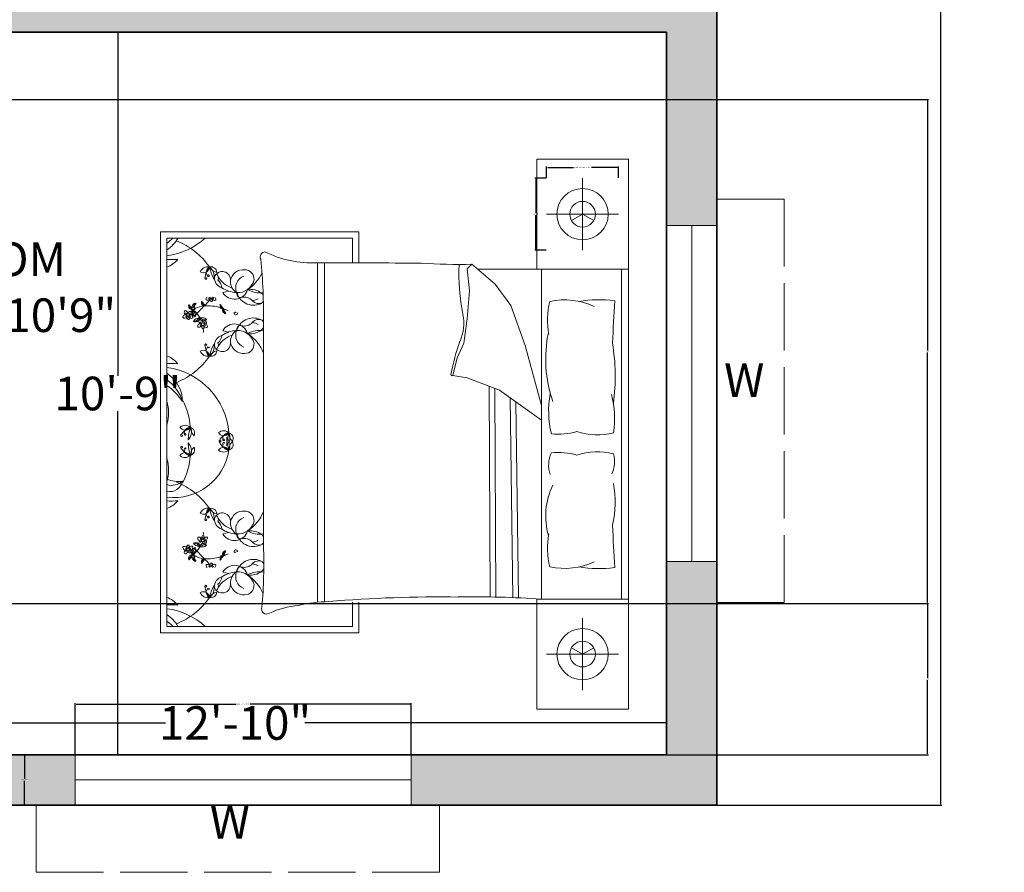
# Model space of a CAD drawing. Units: inches. Extents: x -5 to 482, y -460 to 66.
# Tile 15 of 31: x 306 to 482, y -434 to -282. Entities that reach past the tile are written whole.
import ezdxf

# ---------------------------------------------------------------- set-up
doc = ezdxf.new("R2010")
doc.units = ezdxf.units.IN
doc.header["$MEASUREMENT"] = 0
doc.linetypes.add('ACAD_ISO02W100', pattern=[15, 12, -3])
for name, color, linetype, lineweight in [('A-ANNO-DIMS', 2, 'Continuous', 18), ('A-ANNO-TEXT', 7, 'Continuous', 18), ('A-AREA-IDEN', 7, 'Continuous', 18), ('A-FURN', 8, 'Continuous', 18), ('A-GLAZ', 4, 'Continuous', 18), ('A-GLAZ-OVHD', 4, 'ACAD_ISO02W100', 13), ('A-WALL', 7, 'Continuous', 35), ('A-WALL-PATT', 152, 'Continuous', 13)]:
    doc.layers.add(name, color=color, linetype=linetype, lineweight=lineweight)
doc.styles.get("Standard").update_dxf_attribs({"font": 'arial.ttf'})
doc.dimstyles.get("Standard").update_dxf_attribs({"dimtxt": 0.18, "dimasz": 0.18, "dimexe": 0.18, "dimexo": 0.0625, "dimgap": 0.09, "dimtad": 0, "dimtih": 1, "dimtoh": 1, "dimdec": 0, "dimzin": 0, "dimdsep": 46, "dimlunit": 3, "dimtxsty": 'Standard', "dimcen": 0.09, "dimadec": 0, "dimazin": 0, "dimtfac": 1, "dimtdec": 0, "dimtofl": 0, "dimtmove": 0, "dimatfit": 3, "dimfxl": 1, "dimtolj": 1, "dimtzin": 0, "dimarcsym": 0})

# ---------------------------------------------------------------- blocks, each defined once
blk = doc.blocks.new('*D4')
at = {"layer": 'A-ANNO-DIMS', "color": 0, "lineweight": -2, "transparency": 16777216}
for p, q in [((430.44, 13.15), (470.55, 13.15)), ((470.37, 12.97), (470.37, -201.19)), ((470.37, -421.67), (470.37, -207.5)), ((430.44, -421.85), (470.55, -421.85))]:
    blk.add_line(p, q, dxfattribs=at)
at = {"layer": 'A-ANNO-DIMS', "color": 0, "transparency": 16777216}
for points in [[(470.34, 12.97), (470.4, 12.97), (470.37, 13.15)], [(470.34, -421.67), (470.4, -421.67), (470.37, -421.85)]]:
    blk.add_solid(points, dxfattribs=at)
at = {"layer": 'Defpoints', "color": 0, "transparency": 16777216}
for p in [(430.38, 13.15), (430.38, -421.85), (470.37, -421.85)]:
    blk.add_point(p, dxfattribs=at)
at = {"layer": 'A-ANNO-DIMS', "color": 0, "transparency": 16777216, "insert": (470.37, -204.35), "char_height": 6, "attachment_point": 5}
blk.add_mtext('\\A1;36\'-3"', dxfattribs=at)
blk = doc.blocks.new('*D27')
at = {"layer": 'A-ANNO-DIMS', "color": 0, "lineweight": -2, "transparency": 16777216}
for p, q in [((321.85, -283.85), (323.62, -283.85)), ((323.44, -284.03), (323.44, -345.2)), ((323.44, -412.67), (323.44, -351.5)), ((321.85, -412.85), (323.62, -412.85))]:
    blk.add_line(p, q, dxfattribs=at)
at = {"layer": 'A-ANNO-DIMS', "color": 0, "transparency": 16777216}
for points in [[(323.41, -284.03), (323.47, -284.03), (323.44, -283.85)], [(323.41, -412.67), (323.47, -412.67), (323.44, -412.85)]]:
    blk.add_solid(points, dxfattribs=at)
at = {"layer": 'Defpoints', "color": 0, "transparency": 16777216}
for p in [(321.79, -283.85), (321.79, -412.85), (323.44, -412.85)]:
    blk.add_point(p, dxfattribs=at)
at = {"layer": 'A-ANNO-DIMS', "color": 0, "transparency": 16777216, "insert": (323.44, -348.35), "char_height": 6, "attachment_point": 5}
blk.add_mtext('\\A1;10\'-9"', dxfattribs=at)
blk = doc.blocks.new('*D28')
at = {"layer": 'A-ANNO-DIMS', "color": 0, "lineweight": -2, "transparency": 16777216}
for p, q in [((267.38, -410.79), (267.38, -407)), ((267.56, -407.18), (331.93, -407.18)), ((421.2, -407.18), (356.82, -407.18)), ((421.38, -410.79), (421.38, -407))]:
    blk.add_line(p, q, dxfattribs=at)
at = {"layer": 'A-ANNO-DIMS', "color": 0, "transparency": 16777216}
for points in [[(267.56, -407.15), (267.56, -407.21), (267.38, -407.18)], [(421.2, -407.15), (421.2, -407.21), (421.38, -407.18)]]:
    blk.add_solid(points, dxfattribs=at)
at = {"layer": 'Defpoints', "color": 0, "transparency": 16777216}
for p in [(421.38, -407.18), (267.38, -410.85), (421.38, -410.85)]:
    blk.add_point(p, dxfattribs=at)
at = {"layer": 'A-ANNO-DIMS', "color": 0, "transparency": 16777216, "insert": (344.38, -407.18), "char_height": 6, "attachment_point": 5}
blk.add_mtext('\\A1;12\'-10"', dxfattribs=at)
blk = doc.blocks.new('WIN-GLAZ-60IN')
for p, q in [((0, 9), (60, 9)), ((0, 4.5), (60, 4.5)), ((60, 0), (0, 0))]:
    blk.add_line(p, q)
blk = doc.blocks.new('WIN-SHADE-72IN')
for p, q in [((0, 12), (72, 12)), ((0, 12), (0, 0)), ((72, 12), (72, 0))]:
    blk.add_line(p, q)
blk = doc.blocks.new('BEDSIDE-LAMP-9IN')
for p, q in [((6.42, 12.83), (6.42, 0)), ((0, 6.42), (12.83, 6.42))]:
    blk.add_line(p, q)
for points in [[(6.42, 6.42), (4.43, 7.56)], [(6.42, 6.42), (8.4, 7.56)]]:
    blk.add_lwpolyline(points)
for radius in [4.58, 2.29]:
    blk.add_circle((6.42, 6.42), radius)
blk = doc.blocks.new('*D43')
at = {"layer": 'A-ANNO-DIMS', "color": 0, "lineweight": -2, "transparency": 16777216}
for p, q in [((315.81, -412.79), (315.81, -403.67)), ((315.99, -403.85), (344.59, -403.85)), ((375.63, -403.85), (347.04, -403.85)), ((375.81, -412.79), (375.81, -403.67))]:
    blk.add_line(p, q, dxfattribs=at)
at = {"layer": 'A-ANNO-DIMS', "color": 0, "transparency": 16777216}
for points in [[(315.99, -403.82), (315.99, -403.88), (315.81, -403.85)], [(375.63, -403.82), (375.63, -403.88), (375.81, -403.85)]]:
    blk.add_solid(points, dxfattribs=at)
at = {"layer": 'Defpoints', "color": 0, "transparency": 16777216}
for p in [(375.81, -403.85), (315.81, -412.85), (375.81, -412.85)]:
    blk.add_point(p, dxfattribs=at)
at = {"layer": 'A-ANNO-DIMS', "color": 0, "transparency": 16777216, "insert": (345.81, -403.85), "char_height": 0.18, "attachment_point": 5}
blk.add_mtext('\\A1;WINDOW 5\'-0" TYP.', dxfattribs=at)
blk = doc.blocks.new('*D44')
at = {"layer": 'A-ANNO-DIMS', "color": 0, "lineweight": -2, "transparency": 16777216}
for p, q in [((315.75, -412.85), (306.63, -412.85)), ((306.81, -413.03), (306.81, -417.17)), ((306.81, -421.67), (306.81, -417.53)), ((315.75, -421.85), (306.63, -421.85))]:
    blk.add_line(p, q, dxfattribs=at)
at = {"layer": 'A-ANNO-DIMS', "color": 0, "transparency": 16777216}
for points in [[(306.78, -413.03), (306.84, -413.03), (306.81, -412.85)], [(306.78, -421.67), (306.84, -421.67), (306.81, -421.85)]]:
    blk.add_solid(points, dxfattribs=at)
at = {"layer": 'Defpoints', "color": 0, "transparency": 16777216}
for p in [(306.81, -412.85), (315.81, -412.85), (315.81, -421.85)]:
    blk.add_point(p, dxfattribs=at)
at = {"layer": 'A-ANNO-DIMS', "color": 0, "transparency": 16777216, "insert": (306.81, -417.35), "char_height": 0.18, "attachment_point": 5}
blk.add_mtext('\\A1;0\'-9" TYP.', dxfattribs=at)
blk = doc.blocks.new('*D57')
at = {"layer": 'A-ANNO-DIMS', "color": 0, "lineweight": -2, "transparency": 16777216}
for p, q in [((399.99, -309.85), (399.99, -307.81)), ((400.17, -307.99), (404.81, -307.99)), ((412.64, -307.99), (408, -307.99)), ((412.82, -309.85), (412.82, -307.81))]:
    blk.add_line(p, q, dxfattribs=at)
at = {"layer": 'A-ANNO-DIMS', "color": 0, "transparency": 16777216}
for points in [[(400.17, -307.96), (400.17, -308.02), (399.99, -307.99)], [(412.64, -307.96), (412.64, -308.02), (412.82, -307.99)]]:
    blk.add_solid(points, dxfattribs=at)
at = {"layer": 'Defpoints', "color": 0, "transparency": 16777216}
for p in [(399.99, -307.99), (399.99, -309.91), (412.82, -309.91)]:
    blk.add_point(p, dxfattribs=at)
at = {"layer": 'A-ANNO-DIMS', "color": 0, "transparency": 16777216, "insert": (406.41, -307.99), "char_height": 0.18, "attachment_point": 5}
blk.add_mtext('\\A1;BEDSIDE LAMP 1\'-1" TYP.', dxfattribs=at)
blk = doc.blocks.new('*D58')
at = {"layer": 'A-ANNO-DIMS', "color": 0, "lineweight": -2, "transparency": 16777216}
for p, q in [((399.93, -309.91), (397.88, -309.91)), ((398.06, -310.09), (398.06, -316.15)), ((398.06, -322.57), (398.06, -316.51)), ((399.93, -322.75), (397.88, -322.75))]:
    blk.add_line(p, q, dxfattribs=at)
at = {"layer": 'A-ANNO-DIMS', "color": 0, "transparency": 16777216}
for points in [[(398.03, -310.09), (398.09, -310.09), (398.06, -309.91)], [(398.03, -322.57), (398.09, -322.57), (398.06, -322.75)]]:
    blk.add_solid(points, dxfattribs=at)
at = {"layer": 'Defpoints', "color": 0, "transparency": 16777216}
for p in [(399.99, -309.91), (398.06, -322.75), (399.99, -322.75)]:
    blk.add_point(p, dxfattribs=at)
at = {"layer": 'A-ANNO-DIMS', "color": 0, "transparency": 16777216, "insert": (398.06, -316.33), "char_height": 0.18, "attachment_point": 5}
blk.add_mtext('\\A1;1\'-1" TYP.', dxfattribs=at)
blk = doc.blocks.new('*D74')
at = {"layer": 'A-ANNO-DIMS', "color": 0, "lineweight": -2, "transparency": 16777216}
for p, q in [((214.44, -295.86), (468.16, -295.86)), ((467.98, -296.04), (467.98, -340.68)), ((467.98, -385.68), (467.98, -341.04)), ((214.44, -385.86), (468.16, -385.86))]:
    blk.add_line(p, q, dxfattribs=at)
at = {"layer": 'A-ANNO-DIMS', "color": 0, "transparency": 16777216}
for points in [[(467.95, -296.04), (468.01, -296.04), (467.98, -295.86)], [(467.95, -385.68), (468.01, -385.68), (467.98, -385.86)]]:
    blk.add_solid(points, dxfattribs=at)
at = {"layer": 'Defpoints', "color": 0, "transparency": 16777216}
for p in [(214.38, -295.86), (467.98, -295.86), (214.38, -385.86)]:
    blk.add_point(p, dxfattribs=at)
at = {"layer": 'A-ANNO-DIMS', "color": 0, "transparency": 16777216, "insert": (467.98, -340.86), "char_height": 0.18, "attachment_point": 5}
blk.add_mtext('\\A1;7\'-6"', dxfattribs=at)
blk = doc.blocks.new('*D75')
at = {"layer": 'A-ANNO-DIMS', "color": 0, "lineweight": -2, "transparency": 16777216}
for p, q in [((214.44, -385.86), (468.16, -385.86)), ((467.98, -386.04), (467.98, -399.17)), ((467.98, -412.67), (467.98, -399.54)), ((214.44, -412.85), (468.16, -412.85))]:
    blk.add_line(p, q, dxfattribs=at)
at = {"layer": 'A-ANNO-DIMS', "color": 0, "transparency": 16777216}
for points in [[(467.95, -386.04), (468.01, -386.04), (467.98, -385.86)], [(467.95, -412.67), (468.01, -412.67), (467.98, -412.85)]]:
    blk.add_solid(points, dxfattribs=at)
at = {"layer": 'Defpoints', "color": 0, "transparency": 16777216}
for p in [(214.38, -385.86), (467.98, -385.86), (214.38, -412.85)]:
    blk.add_point(p, dxfattribs=at)
at = {"layer": 'A-ANNO-DIMS', "color": 0, "transparency": 16777216, "insert": (467.98, -399.35), "char_height": 0.18, "attachment_point": 5}
blk.add_mtext('\\A1;2\'-3"', dxfattribs=at)

msp = doc.modelspace()

# ---------------------------------------------------------------- hatches: boundary and pattern name
at = {"layer": 'A-WALL-PATT'}
h = msp.add_hatch(color=256, dxfattribs=at)
h.dxf.hatch_style = 1
h.paths.add_polyline_path([(149.38, -412.85), (144.38, -412.85), (144.38, -283.85), (144.38, -279.35), (133.88, -279.35), (133.88, -283.85), (139.88, -283.85), (139.88, -412.85), (133.51, -412.85), (133.51, -413.92), (102.65, -413.92), (102.65, -421.02), (133.51, -421.02), (133.51, -421.85), (149.38, -421.85)])
h.paths.add_polyline_path([(226.05, -412.85), (218.88, -412.85), (218.88, -350.85), (262.88, -350.85), (262.88, -386.85), (267.38, -386.85), (267.38, -283.85), (270.38, -283.85), (270.38, -279.35), (244.88, -279.35), (244.88, -283.85), (262.88, -283.85), (262.88, -346.35), (218.88, -346.35), (218.88, -283.85), (220.88, -283.85), (220.88, -279.35), (214.38, -279.35), (214.38, -283.85), (214.38, -412.85), (209.38, -412.85), (209.38, -421.85), (226.05, -421.85)])
h.paths.add_polyline_path([(315.81, -412.85), (250.05, -412.85), (250.05, -421.85), (315.81, -421.85)])
h.paths.add_polyline_path([(430.38, -378.35), (421.38, -378.35), (421.38, -412.85), (375.81, -412.85), (375.81, -421.85), (430.38, -421.85)])
h.paths.add_polyline_path([(78.69, -413.92), (47.68, -413.92), (47.68, -412.85), (41.88, -412.85), (41.88, -283.85), (109.88, -283.85), (109.88, -279.35), (41.88, -279.35), (41.88, -241.85), (32.88, -241.85), (32.88, -421.85), (47.68, -421.85), (47.68, -421.02), (78.69, -421.02)])
h.paths.add_polyline_path([(41.88, -144.35), (154.38, -144.35), (154.38, -137.85), (149.88, -137.85), (149.88, -139.85), (41.88, -139.85), (41.88, -97.85), (32.88, -97.85), (32.88, -181.85), (41.88, -181.85)])
h.paths.add_polyline_path([(430.38, -241.85), (421.38, -241.85), (421.38, -279.35), (309.38, -279.35), (309.38, -170.35), (304.88, -170.35), (304.88, -279.35), (294.38, -279.35), (294.38, -283.85), (421.38, -283.85), (421.38, -318.35), (430.38, -318.35)])
h.paths.add_polyline_path([(430.38, -119.85), (421.38, -119.85), (421.38, -139.85), (419.38, -139.85), (419.38, -144.35), (421.38, -144.35), (421.38, -181.85), (430.38, -181.85)])
h.paths.add_polyline_path([(395.38, -139.85), (377.38, -139.85), (377.38, -75.85), (421.38, -75.85), (421.38, -95.85), (430.38, -95.85), (430.38, -45.6), (421.38, -45.6), (421.38, -71.35), (377.38, -71.35), (377.38, -22.85), (372.88, -22.85), (372.88, -139.85), (242.88, -139.85), (242.88, -137.85), (238.38, -137.85), (238.38, -144.35), (304.88, -144.35), (304.88, -146.35), (309.38, -146.35), (309.38, -144.35), (395.38, -144.35)])
h.paths.add_polyline_path([(65.88, 13.15), (32.88, 13.15), (32.88, -37.85), (41.88, -37.85), (41.88, 4.15), (65.88, 4.15)])
h.paths.add_polyline_path([(166.38, 13.15), (125.88, 13.15), (125.88, 4.15), (149.88, 4.15), (149.88, -113.85), (154.38, -113.85), (154.38, 4.15), (166.38, 4.15)])
h.paths.add_polyline_path([(277.88, 13.15), (226.38, 13.15), (226.38, 4.15), (238.38, 4.15), (238.38, -113.85), (242.88, -113.85), (242.88, 4.15), (277.88, 4.15)])
h.paths.add_polyline_path([(430.38, 13.15), (337.88, 13.15), (337.88, 4.15), (372.88, 4.15), (372.88, 1.15), (377.38, 1.15), (377.38, 4.15), (421.38, 4.15), (421.38, -21.6), (430.38, -21.6)])

# ---------------------------------------------------------------- linework, layer by layer
at = {"layer": 'A-FURN'}
for p, q in [((414.59, -306.51), (414.59, -404.72)), ((331.07, -319.47), (366.45, -319.47)), ((331.07, -391.07), (331.07, -319.47)), ((366.45, -319.47), (366.45, -325.03)), ((332.21, -320.61), (332.21, -389.93)), ((365.31, -320.61), (332.21, -320.61)), ((365.31, -325.02), (365.31, -320.61)), ((359.1, -385.62), (359.1, -325.02)), ((360.32, -385.52), (360.32, -325.02)), ((385.81, -326.07), (386.61, -325.27)), ((386.21, -330.04), (385.81, -326.07)), ((386.61, -325.27), (390.78, -328.85)), ((414.59, -326.15), (387.63, -326.15)), ((399.07, -326.15), (399.07, -385.08)), ((413.33, -385.08), (413.33, -326.15)), ((342.16, -330.29), (343.27, -330.07)), ((385.81, -335.02), (386.21, -330.04)), ((390.78, -328.85), (393.57, -332.63)), ((393.57, -332.63), (396.15, -339.79)), ((349.45, -375.55), (349.45, -335.68)), ((385.22, -339.39), (385.81, -335.02)), ((342.16, -337.15), (343.27, -337.37)), ((384.02, -341.98), (385.22, -339.39)), ((396.15, -339.79), (399.07, -350.5)), ((383.23, -345.16), (384.02, -341.98)), ((385.81, -345.56), (383.23, -345.16)), ((391.58, -347.75), (385.81, -345.56)), ((389.88, -384.73), (389.73, -347.05)), ((390.89, -384.72), (390.74, -347.43)), ((399.07, -353.13), (391.58, -347.75)), ((393.98, -384.77), (393.48, -349.11)), ((394.99, -384.81), (394.5, -349.85)), ((342.16, -373.39), (343.27, -373.17)), ((342.16, -380.25), (343.27, -380.47)), ((365.31, -389.93), (365.31, -385.6)), ((366.45, -385.62), (366.45, -391.07)), ((332.21, -389.93), (365.31, -389.93)), ((366.45, -391.07), (331.07, -391.07))]:
    msp.add_line(p, q, dxfattribs=at)
for points in [[(398.22, -326.15), (398.22, -306.51), (414.59, -306.51)], [(414.59, -385.08), (398.22, -385.08), (398.22, -404.72), (414.59, -404.72)]]:
    msp.add_lwpolyline(points, dxfattribs=at)
for points in [[(377.62, -325.07, 0.001242), (358.98, -325.02, -0.127202), (349.7, -323.05)], [(412.14, -331.79, 0.074897), (405.73, -331.91, -0.472817)], [(405.37, -355.15, 0.14099), (411.91, -355.35, 0.235245)], [(405.37, -359.35, -0.14099), (411.91, -359.15, -0.235245)], [(412.14, -379.44, -0.074897), (405.73, -379.32, 0.472817)], [(361.1, -385.5, 0.056112), (355.69, -386.21, 0.095341), (350.49, -387.59)]]:
    msp.add_lwpolyline(points, format="xyb", dxfattribs=at)
for centre in [(335.97, -334.32), (338.61, -335.96), (338.61, -374.58), (335.97, -376.22)]:
    msp.add_circle(centre, 0.25, dxfattribs=at)
for centre, radius, start, end in [((327.6, -315.25), 7.79, 306.3036, 316.4814), ((328.76, -317.49), 6.25, 303.4617, 330.1116), ((330.48, -311.06), 12.82, 277.745, 311.8856), ((329.21, -333), 12.82, 34.3865, 68.5908), ((349.76, -323.95), 0.906, 93.98, 207.3412), ((330.21, -320.99), 5.21, 292.5547, 318.9546), ((333.01, -306.71), 17.74, 267.4081, 273.6519), ((247.22, -334.5), 102.24, 359.3433, 5.6887), ((384.17, -235.22), 90.08, 265.8294, 271.553), ((339.49, -327.15), 1.42, 77.7115, 159.0387), ((338.72, -325.73), 1.07, 238.4633, 358.2869), ((342.24, -327.89), 3.24, 138.8402, 177.9352), ((340.28, -326.69), 1.05, 117.6827, 223.7762), ((340.05, -326.79), 1.06, 2.9516, 103.728), ((348.55, -323.81), 8.97, 192.5173, 207.1824), ((338.61, -327.4), 2.03, 345.4653, 54.2343), ((341.66, -324.62), 2.19, 211.3827, 255.2969), ((342.08, -328.04), 1.47, 350.264, 160.8688), ((345.87, -328.58), 2.35, 84.9449, 172.8857), ((346.1, -327.9), 1.66, 354.4856, 91.0538), ((421.39, -326.95), 37.07, 177.4519, 191.3392), ((339.15, -327.78), 0.159, 177.9352, 11.4834), ((339.23, -327.77), 0.0774, 11.4834, 127.9409), ((339.62, -327.32), 0.139, 223.7762, 159.7183), ((342.53, -327.69), 1.84, 175.969, 254.3045), ((340.49, -327.74), 0.903, 333.9755, 53.2681), ((340.08, -329.67), 1.96, 6.1662, 51.5825), ((345.33, -325.12), 4.64, 211.2614, 251.7045), ((346.39, -328.17), 2.85, 182.3591, 234.0401), ((346.76, -329.5), 2.28, 111.5819, 201.4221), ((344.88, -327.39), 2.95, 265.2933, 346.921), ((342.53, -323.57), 7.43, 303.6671, 333.2997), ((344.95, -325.07), 5.27, 236.2883, 266.5076), ((344.28, -329.07), 2.44, 209.9085, 343.1337), ((346.96, -333.53), 3.79, 122.7011, 126.3445), ((348.72, -326.3), 4.07, 238.8218, 279.1554), ((346.96, -333.53), 3.79, 55.785, 94.7304), ((348.36, -331.34), 1.18, 30.0293, 52.325), ((341.14, -331.95), 2.77, 178.3264, 187.1302), ((338.15, -332.33), 0.516, 11.3256, 64.4621), ((339.9, -331.59), 1.55, 190.2588, 210.656), ((332.52, -325.89), 9.32, 313.1541, 322.0459), ((339.38, -331.49), 0.192, 142.4737, 265.053), ((339.63, -331.45), 0.413, 127.7621, 169.0403), ((339.41, -331.1), 0.581, 265.053, 338.3618), ((340.18, -331.9), 0.759, 113.4276, 137.6104), ((340.09, -331.11), 0.25, 183.2768, 356.7232), ((340.28, -331.56), 0.409, 139.7889, 227.6792), ((340.14, -331.71), 0.216, 227.6792, 350.3487), ((339.31, -331.56), 0.819, 353.0852, 15.7171), ((339.85, -331.66), 0.517, 350.3487, 43.6538), ((340.81, -331.12), 0.601, 198.7263, 262.5032), ((340.33, -331.4), 0.239, 1.1081, 91.8675), ((340.48, -331.46), 0.417, 11.5637, 52.6358), ((340.78, -331.53), 0.193, 255.2356, 54.9248), ((345.31, -330.62), 0.61, 167.3041, 285.1471), ((347.67, -329.45), 3.13, 199.2822, 299.1751), ((345.99, -333.15), 2.01, 41.5653, 105.1471), ((347.1, -328.98), 2.82, 277.436, 299.9149), ((348.6, -330.84), 1.47, 221.5653, 293.8354), ((348.36, -331.34), 1.18, 314.4517, 333.558), ((413.29, -335.29), 13.16, 165.1039, 191.0369), ((403.15, -344.3), 12.66, 65.1316, 101.7583), ((1346.78, -385.92), 936.2, 176.68521, 177.14978), ((335.78, -333.82), 0.494, 157.4086, 261.4386), ((335.5, -333.8), 0.248, 58.0499, 135.6268), ((335.21, -334.26), 0.789, 14.7558, 58.0499), ((336.32, -334.05), 0.341, 36.1046, 181.4281), ((336.33, -332.71), 0.279, 124.3538, 214.3923), ((336.74, -332.75), 0.651, 190.3057, 287.1958), ((336.93, -332.52), 0.756, 176.9701, 248.2913), ((342.33, -328.54), 7.31, 212.6784, 216.3746), ((336.41, -334.01), 0.245, 263.7526, 41.7054), ((336.68, -332.7), 0.289, 216.3746, 291.7548), ((339.23, -336.76), 4.08, 124.0033, 132.4917), ((335.04, -337.27), 4.36, 63.7819, 68.2913), ((337.37, -333.92), 0.693, 128.3208, 208.8162), ((337.37, -332.9), 0.651, 122.8155, 187.3992), ((336.86, -333.17), 0.218, 289.3605, 111.7548), ((337.03, -333.17), 0.218, 221.8703, 44.2646), ((338.02, -333.8), 1.14, 157.2305, 229.0635), ((337.65, -332.98), 0.756, 109.4799, 177.6828), ((337.63, -333.43), 0.671, 174.4544, 220.6188), ((333.82, -337.18), 4.89, 30.544, 49.818), ((337.25, -332.5), 0.279, 56.8636, 146.9021), ((337.39, -332.82), 0.289, 148.8844, 224.2646), ((336.51, -334.39), 0.806, 340.0041, 40.6188), ((343.4, -336.44), 7.31, 145.1882, 148.8844), ((339.23, -336.76), 4.08, 94.756, 119.2041), ((347.92, -342.63), 13.42, 132.2412, 142.1744), ((338.86, -332.22), 0.471, 188.3432, 274.2869), ((339.27, -331.96), 0.823, 210.656, 242.6341), ((339.9, -331.25), 1.58, 218.2101, 226.3071), ((338.73, -332.58), 0.2, 325.7657, 67.4417), ((339.44, -340.81), 8.13, 73.5842, 93.8277), ((344.45, -332.53), 2.77, 178.3264, 187.1302), ((341.46, -332.92), 0.516, 11.3256, 64.4621), ((343.21, -332.17), 1.55, 190.2588, 210.656), ((342.17, -332.81), 0.471, 188.3432, 274.2869), ((342.58, -332.55), 0.823, 210.656, 242.6341), ((343.2, -331.84), 1.58, 218.2101, 226.3071), ((342.03, -333.16), 0.2, 325.7657, 67.4417), ((342.6, -333.53), 0.471, 147.5332, 233.4768), ((343.02, -333.29), 0.823, 179.1859, 211.164), ((342.22, -333.48), 0.2, 354.3784, 96.0543), ((339.44, -340.81), 8.13, 63.0032, 69.8941), ((343.65, -332.91), 1.55, 211.164, 231.5612), ((343.92, -331.65), 2.77, 234.6898, 243.4936), ((343.94, -333.07), 1.58, 195.5129, 203.6099), ((342.17, -334.1), 0.516, 357.3579, 50.4944), ((344.38, -334), 0.189, 12.7051, 190.4384), ((344.5, -333.98), 0.308, 190.4384, 10.4136), ((335.25, -334.7), 0.192, 142.4737, 265.053), ((335.51, -334.67), 0.413, 61.2196, 169.0403), ((335.29, -334.32), 0.581, 265.053, 338.3618), ((336.06, -335.11), 0.759, 113.4276, 137.6104), ((335.76, -333.95), 0.166, 172.906, 277.132), ((336.15, -334.78), 0.409, 139.7889, 227.6792), ((336.02, -334.92), 0.216, 227.6792, 350.3487), ((335.19, -334.77), 0.819, 353.0852, 15.7171), ((335.73, -334.87), 0.517, 350.3487, 43.6538), ((336.68, -334.34), 0.601, 198.7263, 262.5032), ((336.12, -333.78), 0.344, 270.0645, 331.1507), ((336.41, -333.86), 0.393, 221.8413, 265.7877), ((336.21, -334.62), 0.239, 1.1081, 91.8675), ((336.36, -334.67), 0.417, 11.5637, 86.365), ((336.65, -334.75), 0.193, 255.2356, 54.9248), ((337.49, -333.87), 0.828, 207.7043, 254.3516), ((336.95, -334.34), 1.14, 270.278, 342.111), ((337.71, -335.77), 0.806, 98.7227, 159.3375), ((337.31, -334.73), 0.828, 244.9899, 291.6373), ((337.49, -334.31), 0.671, 278.7227, 324.8872), ((337.37, -334.85), 0.693, 290.5253, 358.5375), ((338.41, -335.45), 0.494, 157.4086, 261.4386), ((338.14, -335.44), 0.248, 58.0499, 135.6268), ((338.72, -334.65), 0.693, 182.8499, 266.1226), ((338.45, -334.17), 0.671, 231.7607, 277.9252), ((338.98, -334.05), 1.14, 214.5369, 286.3699), ((338.39, -335.59), 0.166, 172.906, 277.132), ((337.85, -335.89), 0.789, 14.7558, 58.0499), ((333.82, -337.18), 4.89, 23.0501, 23.8477), ((338.66, -335.63), 0.806, 37.3105, 97.9252), ((338.95, -335.68), 0.341, 36.1046, 181.4281), ((338.75, -334.52), 0.828, 265.0106, 311.658), ((338.75, -335.42), 0.344, 270.0645, 331.1507), ((339.05, -335.65), 0.245, 263.7526, 41.7054), ((347.67, -337.99), 3.13, 60.8249, 160.7178), ((345.99, -334.29), 2.01, 254.8529, 318.4347), ((347.1, -338.46), 2.82, 60.0851, 82.564), ((348.6, -336.6), 1.47, 66.1646, 138.4347), ((348.36, -336.1), 1.18, 23.229, 45.5483), ((377.21, -335.81), 7.99, 336.2616, 11.3392), ((337.89, -336.34), 0.192, 142.4737, 265.053), ((338.14, -336.3), 0.413, 61.2196, 169.0403), ((337.92, -335.95), 0.581, 265.053, 338.3618), ((338.69, -336.75), 0.759, 113.4276, 137.6104), ((338.79, -336.41), 0.409, 139.7889, 227.6792), ((338.66, -336.56), 0.216, 227.6792, 350.3487), ((337.82, -336.41), 0.819, 353.0852, 15.7171), ((333.82, -337.18), 4.89, 357.1071, 4.7585), ((338.36, -336.51), 0.517, 350.3487, 43.6538), ((339.05, -335.5), 0.393, 221.8413, 265.7877), ((339.32, -335.97), 0.601, 198.7263, 262.5032), ((338.84, -336.25), 0.239, 1.1081, 91.8675), ((338.99, -336.31), 0.417, 11.5637, 86.365), ((339.29, -336.38), 0.193, 255.2356, 54.9248), ((344.95, -342.36), 5.27, 93.4924, 123.7117), ((344.28, -338.37), 2.44, 16.8663, 150.0915), ((346.39, -339.27), 2.85, 125.9599, 177.6409), ((346.76, -337.93), 2.28, 158.5779, 248.4181), ((344.88, -340.05), 2.95, 13.079, 94.7067), ((345.31, -336.82), 0.61, 74.8529, 192.6959), ((346.96, -333.91), 3.79, 233.6555, 237.2989), ((348.72, -341.14), 4.07, 79.7133, 121.1782), ((346.96, -333.91), 3.79, 265.2696, 304.215), ((348.36, -336.1), 1.18, 307.675, 336.7144), ((342.53, -339.75), 1.84, 105.6955, 184.031), ((342.08, -339.4), 1.47, 199.1312, 9.736), ((340.08, -337.77), 1.96, 308.4175, 353.8338), ((345.33, -342.32), 4.64, 108.2955, 148.7386), ((345.87, -338.86), 2.35, 187.1143, 275.0551), ((342.53, -343.87), 7.43, 21.4941, 56.3329), ((420.34, -351.98), 38.09, 160.1194, 169.3383), ((422.65, -342.22), 22.83, 168.0397, 199.2615), ((338.72, -341.71), 1.07, 1.7131, 121.5367), ((339.49, -340.29), 1.42, 200.9613, 282.2885), ((339.15, -339.65), 0.159, 348.5166, 182.0648), ((342.24, -339.54), 3.24, 182.0648, 221.1598), ((339.23, -339.67), 0.0774, 232.0591, 348.5166), ((340.28, -340.75), 1.05, 136.2238, 242.3173), ((339.68, -340.13), 0.0836, 200.2667, 136.2271), ((338.61, -340.03), 2.03, 305.7657, 14.5347), ((348.55, -343.62), 8.97, 152.8176, 167.4827), ((340.05, -340.65), 1.06, 256.272, 357.0484), ((341.66, -342.82), 2.19, 104.7031, 148.6173), ((340.49, -339.7), 0.903, 306.7319, 26.0245), ((346.1, -339.54), 1.66, 268.9462, 5.5144), ((376.6, -345.25), 35.62, 352.2196, 9.497), ((330.21, -346.44), 5.21, 41.0454, 67.4453), ((329.21, -334.44), 12.82, 291.4092, 325.6135), ((333.01, -360.73), 17.74, 86.3481, 92.5919), ((330.48, -356.38), 12.82, 4.4623, 82.255), ((328.76, -349.94), 6.25, 1.272, 56.5383), ((327.6, -352.19), 7.79, 17.8504, 53.6964), ((383.15, -344.94), 0.237, 178.8623, 289.7536), ((325.41, -356.28), 11.58, 34.0123, 54.053), ((325.46, -351.81), 7.05, 343.5431, 17.0202), ((323.61, -355.39), 12.82, 4.4623, 27.4146), ((417.66, -351.46), 17.32, 169.8617, 193.6238), ((394.6, -352.77), 17.5, 351.5249, 13.96), ((321.83, -354.6), 10.43, 4.3787, 5.6357), ((314.69, -360.09), 18.64, 19.7217, 19.9028), ((335.44, -355.45), 1.42, 47.7873, 129.1145), ((335.48, -353.83), 1.07, 208.5391, 328.3627), ((337.45, -357.47), 3.24, 108.9159, 148.011), ((336.35, -355.45), 1.05, 87.7585, 193.852), ((344.96, -357.08), 8.97, 162.593, 177.2582), ((334.55, -355.23), 2.03, 315.5411, 24.3101), ((338.59, -354.34), 2.19, 181.4585, 225.3727), ((336.1, -355.42), 1.06, 333.0274, 73.8037), ((342.31, -356.43), 1.42, 47.7873, 129.1145), ((334.83, -355.83), 0.159, 148.011, 341.5592), ((334.91, -355.86), 0.0774, 341.5592, 98.0167), ((335.47, -355.66), 0.139, 193.852, 129.9245), ((342.35, -354.82), 1.07, 208.5391, 328.3627), ((341.7, -356.81), 0.159, 148.011, 341.5592), ((344.32, -358.45), 3.24, 108.9159, 148.011), ((341.78, -356.84), 0.0774, 341.5592, 98.0167), ((343.22, -356.43), 1.05, 87.7585, 193.852), ((342.34, -356.64), 0.139, 193.852, 129.9245), ((341.42, -356.21), 2.03, 315.5411, 24.3101), ((351.83, -358.06), 8.97, 162.593, 177.2582), ((341.42, -357.6), 2.03, 335.6899, 44.4589), ((351.83, -355.75), 8.97, 182.7418, 197.407), ((342.97, -356.4), 1.06, 333.0274, 73.8037), ((345.45, -355.32), 2.19, 181.4585, 225.3727), ((402.09, -343.58), 12.03, 264.0129, 285.8293), ((333.44, -357.02), 9.93, 262.8636, 351.8197), ((334.83, -357.98), 0.159, 18.4408, 211.989), ((337.45, -356.35), 3.24, 211.989, 251.0841), ((334.91, -357.96), 0.0774, 261.9833, 18.4408), ((336.35, -358.37), 1.05, 166.148, 272.2415), ((335.52, -358.14), 0.0836, 230.1909, 166.0209), ((344.96, -356.73), 8.97, 182.7418, 197.407), ((334.55, -358.58), 2.03, 335.6899, 44.4589), ((338.59, -359.47), 2.19, 134.6273, 178.5415), ((336.1, -358.4), 1.06, 286.1963, 26.9726), ((342.35, -359), 1.07, 31.6373, 151.4609), ((342.31, -357.38), 1.42, 230.8855, 312.2127), ((341.7, -357), 0.159, 18.4408, 211.989), ((344.32, -355.37), 3.24, 211.989, 251.0841), ((341.78, -356.98), 0.0774, 261.9833, 18.4408), ((343.22, -357.39), 1.05, 166.148, 272.2415), ((342.39, -357.16), 0.0836, 230.1909, 166.0209), ((342.97, -357.41), 1.06, 286.1963, 26.9726), ((345.45, -358.49), 2.19, 134.6273, 178.5415), ((325.46, -362.01), 7.05, 342.9798, 16.4569), ((321.83, -359.21), 10.43, 354.3643, 355.6213), ((314.69, -353.72), 18.64, 340.0972, 340.2783), ((335.48, -359.98), 1.07, 31.6373, 151.4609), ((335.44, -358.36), 1.42, 230.8855, 312.2127), ((323.61, -358.42), 12.82, 332.5854, 355.5377), ((405.55, -361.15), 5.21, 155.0183, 198.5407), ((402.09, -370.92), 12.03, 74.1707, 95.9871), ((407.25, -360.5), 4.86, 333.3437, 16.1026), ((334.35, -358.31), 5.74, 248.117, 276.6195), ((332.75, -363.57), 2.3, 256.3898, 349.0739), ((333.06, -361.84), 2.91, 252.8609, 311.9049), ((329.21, -376.11), 12.82, 34.3865, 68.5908), ((412.32, -370.25), 12.5, 153.8761, 196.1746), ((394.96, -367.78), 17.26, 346.3427, 11.1841), ((333.01, -349.81), 17.74, 267.4081, 273.6519), ((330.21, -364.1), 5.21, 292.5547, 318.9546), ((339.49, -370.25), 1.42, 77.7115, 159.0387), ((338.72, -368.83), 1.07, 238.4633, 358.2869), ((342.24, -371), 3.24, 138.8402, 177.9352), ((340.28, -369.79), 1.05, 117.6827, 223.7762), ((340.05, -369.9), 1.06, 2.9516, 103.728), ((341.66, -367.72), 2.19, 211.3827, 255.2969), ((338.61, -370.51), 2.03, 345.4653, 54.2343), ((348.55, -366.92), 8.97, 192.5173, 207.1824), ((339.23, -370.87), 0.0774, 11.4834, 127.9409), ((339.62, -370.42), 0.139, 223.7762, 159.7183), ((342.08, -371.14), 1.47, 350.264, 160.8688), ((342.53, -370.79), 1.84, 175.969, 254.3045), ((340.49, -370.84), 0.903, 333.9755, 53.2681), ((345.33, -368.22), 4.64, 211.2614, 251.7045), ((345.87, -371.68), 2.35, 84.9449, 172.8857), ((346.76, -372.61), 2.28, 111.5819, 201.4221), ((346.1, -371), 1.66, 354.4856, 91.0538), ((342.53, -366.67), 7.43, 303.6671, 338.5059), ((339.15, -370.89), 0.159, 177.9352, 11.4834), ((340.08, -372.77), 1.96, 6.1662, 51.5825), ((344.95, -368.18), 5.27, 236.2883, 266.5076), ((346.39, -371.28), 2.85, 182.3591, 234.0401), ((344.88, -370.49), 2.95, 265.2933, 346.921), ((1346.78, -325.3), 936.2, 182.85022, 183.31479), ((337.89, -374.2), 0.192, 94.947, 217.5263), ((338.14, -374.24), 0.413, 190.9597, 298.7804), ((337.92, -374.59), 0.581, 21.6382, 94.947), ((338.69, -373.79), 0.759, 222.3896, 246.5724), ((338.79, -374.13), 0.409, 132.3208, 220.2111), ((338.66, -373.98), 0.216, 9.6513, 132.3208), ((337.82, -374.13), 0.819, 344.2829, 6.9148), ((333.82, -373.37), 4.89, 355.2415, 2.8929), ((338.36, -374.03), 0.517, 316.3462, 9.6513), ((339.32, -374.57), 0.601, 97.4968, 161.2737), ((338.84, -374.29), 0.239, 268.1325, 358.8919), ((338.99, -374.23), 0.417, 273.635, 348.4363), ((339.29, -374.16), 0.193, 305.0752, 104.7644), ((344.28, -372.17), 2.44, 209.9085, 343.1337), ((345.31, -373.72), 0.61, 167.3041, 285.1471), ((346.96, -376.64), 3.79, 122.7011, 126.3445), ((347.67, -372.55), 3.13, 199.2822, 299.1751), ((345.99, -376.25), 2.01, 41.5653, 105.1471), ((348.72, -369.4), 4.07, 238.8218, 280.2867), ((346.96, -376.64), 3.79, 55.785, 94.7304), ((348.36, -374.44), 1.18, 23.2856, 52.325), ((413.29, -375.93), 13.16, 168.9631, 194.8961), ((335.25, -375.84), 0.192, 94.947, 217.5263), ((335.51, -375.88), 0.413, 190.9597, 298.7804), ((335.29, -376.22), 0.581, 21.6382, 94.947), ((336.06, -375.43), 0.759, 222.3896, 246.5724), ((336.15, -375.76), 0.409, 132.3208, 220.2111), ((336.02, -375.62), 0.216, 9.6513, 132.3208), ((335.19, -375.77), 0.819, 344.2829, 6.9148), ((335.73, -375.67), 0.517, 316.3462, 9.6513), ((336.68, -376.2), 0.601, 97.4968, 161.2737), ((336.21, -375.92), 0.239, 268.1325, 358.8919), ((336.36, -375.87), 0.417, 273.635, 348.4363), ((336.65, -375.8), 0.193, 305.0752, 104.7644), ((337.49, -376.67), 0.828, 105.6484, 152.2957), ((338.02, -376.74), 1.14, 130.9365, 202.7695), ((337.31, -375.81), 0.828, 68.3627, 115.0101), ((336.95, -376.2), 1.14, 17.889, 89.722), ((337.71, -374.77), 0.806, 200.6625, 261.2773), ((333.82, -373.37), 4.89, 310.182, 329.456), ((336.51, -376.15), 0.806, 319.3812, 19.9959), ((337.49, -376.23), 0.671, 35.1128, 81.2773), ((337.37, -375.69), 0.693, 1.4625, 69.4747), ((338.41, -375.09), 0.494, 98.5614, 202.5914), ((338.14, -375.11), 0.248, 224.3732, 301.9501), ((338.72, -375.89), 0.693, 93.8774, 177.1501), ((338.98, -376.49), 1.14, 73.6301, 145.4631), ((338.45, -376.38), 0.671, 82.0748, 128.2393), ((338.39, -374.95), 0.166, 82.868, 187.094), ((337.85, -374.65), 0.789, 301.9501, 345.2442), ((333.82, -373.37), 4.89, 336.1523, 336.9499), ((338.66, -374.91), 0.806, 262.0748, 322.6895), ((338.95, -374.86), 0.341, 178.5719, 323.8954), ((338.75, -376.02), 0.828, 48.342, 94.9894), ((339.05, -375.04), 0.393, 94.2123, 138.1587), ((338.75, -375.12), 0.344, 28.8493, 89.9355), ((339.05, -374.89), 0.245, 318.2946, 96.2474), ((347.1, -372.08), 2.82, 277.436, 299.9149), ((348.6, -373.94), 1.47, 221.5653, 293.8354), ((253.93, -378.56), 95.57, 355.2402, 1.8035), ((348.36, -374.44), 1.18, 314.4517, 336.7144), ((335.78, -376.73), 0.494, 98.5614, 202.5914), ((335.5, -376.74), 0.248, 224.3732, 301.9501), ((335.76, -376.59), 0.166, 82.868, 187.094), ((335.21, -376.28), 0.789, 301.9501, 345.2442), ((336.32, -376.49), 0.341, 178.5719, 323.8954), ((336.33, -377.83), 0.279, 145.6077, 235.6462), ((336.74, -377.79), 0.651, 72.8042, 169.6943), ((336.41, -376.68), 0.393, 94.2123, 138.1587), ((336.12, -376.76), 0.344, 28.8493, 89.9355), ((336.93, -378.02), 0.756, 111.7087, 183.0299), ((342.33, -382), 7.31, 143.6254, 147.3216), ((336.41, -376.53), 0.245, 318.2946, 96.2474), ((336.68, -377.84), 0.289, 68.2452, 143.6254), ((339.23, -373.78), 4.08, 227.5083, 235.9967), ((335.04, -373.27), 4.36, 291.7087, 296.2181), ((337.37, -376.62), 0.693, 151.1838, 231.6792), ((337.37, -377.64), 0.651, 172.6008, 237.1845), ((336.86, -377.37), 0.218, 248.2452, 70.6395), ((337.03, -377.37), 0.218, 315.7354, 138.1297), ((337.65, -377.56), 0.756, 182.3172, 250.5201), ((337.63, -377.11), 0.671, 139.3812, 185.5456), ((337.39, -377.72), 0.289, 135.7354, 211.1156), ((339.23, -373.78), 4.08, 240.7959, 265.244), ((347.92, -367.91), 13.42, 217.8256, 227.7588), ((338.86, -378.32), 0.471, 85.7131, 171.6568), ((339.27, -378.58), 0.823, 117.3659, 149.344), ((338.73, -377.96), 0.2, 292.5583, 34.2343), ((339.44, -369.73), 8.13, 266.1723, 286.4158), ((332.52, -384.65), 9.32, 37.9541, 46.8459), ((343.21, -378.37), 1.55, 149.344, 169.7412), ((344.45, -378.01), 2.77, 172.8698, 181.6736), ((341.46, -377.62), 0.516, 295.5379, 348.6744), ((342.17, -377.73), 0.471, 85.7131, 171.6568), ((342.58, -377.99), 0.823, 117.3659, 149.344), ((343.2, -378.7), 1.58, 133.6929, 141.7899), ((342.03, -377.38), 0.2, 292.5583, 34.2343), ((342.6, -377.01), 0.471, 126.5232, 212.4668), ((343.02, -377.25), 0.823, 148.836, 180.8141), ((342.22, -377.06), 0.2, 263.9457, 5.6216), ((339.44, -369.73), 8.13, 290.1059, 296.9968), ((343.65, -377.63), 1.55, 128.4388, 148.836), ((343.92, -378.89), 2.77, 116.5064, 125.3102), ((343.94, -377.47), 1.58, 156.3901, 164.4871), ((342.17, -376.44), 0.516, 309.5056, 2.6421), ((344.38, -376.54), 0.189, 169.5616, 347.2949), ((344.5, -376.56), 0.308, 349.5864, 169.5616), ((337.25, -378.04), 0.279, 213.0979, 303.1364), ((343.4, -374.1), 7.31, 211.1156, 214.8118), ((339.9, -378.95), 1.55, 149.344, 169.7412), ((341.14, -378.59), 2.77, 172.8698, 181.6736), ((338.15, -378.21), 0.516, 295.5379, 348.6744), ((339.9, -379.29), 1.58, 133.6929, 141.7899), ((339.38, -379.05), 0.192, 94.947, 217.5263), ((339.63, -379.09), 0.413, 190.9597, 232.2379), ((339.41, -379.44), 0.581, 21.6382, 94.947), ((340.18, -378.64), 0.759, 222.3896, 246.5724), ((340.09, -379.43), 0.25, 3.2768, 176.7232), ((340.28, -378.98), 0.409, 132.3208, 220.2111), ((340.14, -378.83), 0.216, 9.6513, 132.3208), ((339.31, -378.98), 0.819, 344.2829, 6.9148), ((339.85, -378.88), 0.517, 316.3462, 9.6513), ((340.81, -379.42), 0.601, 97.4968, 161.2737), ((340.33, -379.14), 0.239, 268.1325, 358.8919), ((340.78, -379.01), 0.193, 305.0752, 104.7644), ((340.48, -379.08), 0.417, 307.3642, 348.4363), ((344.28, -381.47), 2.44, 16.8663, 150.0915), ((345.31, -379.93), 0.61, 74.8529, 192.6959), ((347.67, -381.09), 3.13, 60.8249, 160.7178), ((345.99, -377.39), 2.01, 254.8529, 318.4347), ((347.1, -381.57), 2.82, 60.0851, 82.564), ((348.6, -379.7), 1.47, 66.1646, 138.4347), ((348.36, -379.2), 1.18, 307.675, 342.5814), ((348.36, -379.2), 1.18, 16.6343, 45.5483), ((403.15, -366.92), 12.66, 258.2417, 294.8684), ((342.53, -382.85), 1.84, 105.6955, 184.031), ((340.08, -380.87), 1.96, 308.4175, 353.8338), ((345.33, -385.42), 4.64, 108.2955, 148.7386), ((344.95, -385.47), 5.27, 93.4924, 123.7117), ((346.39, -382.37), 2.85, 125.9599, 177.6409), ((346.76, -381.04), 2.28, 158.5779, 248.4181), ((344.88, -383.15), 2.95, 13.079, 94.7067), ((346.96, -377.01), 3.79, 233.6555, 237.2989), ((348.72, -384.24), 4.07, 79.249, 121.1782), ((346.96, -377.01), 3.79, 265.2696, 304.215), ((342.53, -386.97), 7.43, 23.6453, 56.3329), ((339.15, -382.76), 0.159, 348.5166, 182.0648), ((342.24, -382.65), 3.24, 182.0648, 221.1598), ((339.23, -382.77), 0.0774, 232.0591, 348.5166), ((340.28, -383.85), 1.05, 136.2238, 242.3173), ((348.55, -386.73), 8.97, 152.8176, 167.4827), ((338.61, -383.14), 2.03, 305.7657, 14.5347), ((342.08, -382.5), 1.47, 199.1312, 9.736), ((340.49, -382.8), 0.903, 306.7319, 26.0245), ((345.87, -381.96), 2.35, 187.1143, 275.0551), ((346.1, -382.64), 1.66, 268.9462, 5.5144), ((330.21, -389.55), 5.21, 41.0454, 67.4453), ((329.21, -377.54), 12.82, 291.4092, 325.6135), ((338.72, -384.81), 1.07, 1.7131, 121.5367), ((339.49, -383.39), 1.42, 200.9613, 282.2885), ((339.68, -383.24), 0.0836, 200.2667, 136.2271), ((341.66, -385.92), 2.19, 104.7031, 148.6173), ((340.05, -383.75), 1.06, 256.272, 357.0484), ((380.65, -614.86), 230.19, 89.1145, 94.8735), ((387.07, -561.13), 176.47, 86.1, 90.9282), ((333.01, -403.83), 17.74, 86.3481, 92.5919), ((349.99, -386.84), 0.895, 156.5219, 303.8264), ((330.48, -399.48), 12.82, 48.1144, 82.255), ((328.76, -393.05), 6.25, 29.8884, 56.5383), ((327.6, -395.29), 7.79, 43.5186, 53.6964)]:
    msp.add_arc(centre, radius, start, end, dxfattribs=at)
at = {"layer": 'A-GLAZ'}
for p, q in [((430.38, -318.35), (421.38, -318.35)), ((421.38, -378.35), (430.38, -378.35)), ((315.81, -421.85), (315.81, -412.85)), ((375.81, -412.85), (375.81, -421.85))]:
    msp.add_line(p, q, dxfattribs=at)
at = {"layer": 'A-WALL'}
for p, q in [((430.38, 13.15), (430.38, -421.85)), ((294.38, -283.85), (421.38, -283.85)), ((421.38, -283.85), (421.38, -412.85)), ((218.88, -412.85), (421.38, -412.85)), ((133.51, -421.85), (430.38, -421.85))]:
    msp.add_line(p, q, dxfattribs=at)

# ---------------------------------------------------------------- block references
at = {"layer": 'A-FURN', "rotation": 180}
msp.add_blockref('BEDSIDE-LAMP-9IN', (412.82, -309.91), dxfattribs=at)
at = {"layer": 'A-FURN'}
msp.add_blockref('BEDSIDE-LAMP-9IN', (399.99, -401.31), dxfattribs=at)
at = {"layer": 'A-GLAZ', "rotation": 90.00000000000003}
msp.add_blockref('WIN-GLAZ-60IN', (430.38, -378.35), dxfattribs=at)
at = {"layer": 'A-GLAZ'}
msp.add_blockref('WIN-GLAZ-60IN', (315.82, -421.85), dxfattribs=at)
at = {"layer": 'A-GLAZ-OVHD'}
for p, rotation in [((430.38, -313.66), 270), ((380.87, -421.85), 180)]:
    msp.add_blockref('WIN-SHADE-72IN', p, dxfattribs=dict(at, rotation=rotation))

# ---------------------------------------------------------------- texts
at = {"layer": 'A-ANNO-TEXT', "char_height": 6, "attachment_point": 1}
for insert in [(431.66, -342.96), (339.84, -421.85)]:
    msp.add_mtext('W', dxfattribs=dict(at, insert=insert))
at = {"layer": 'A-AREA-IDEN', "insert": (274.34, -321.37), "char_height": 6, "attachment_point": 1}
msp.add_mtext('BEDROOM\\P12\'10"X10\'9"', dxfattribs=at)

# ---------------------------------------------------------------- dimensions: what is measured, and where the dimension line sits
at = {"layer": 'A-ANNO-DIMS'}
for base, p1, p2, override, picture, middle in [((470.37, -421.85), (430.38, 13.15), (430.38, -421.85), {"dimtxt": 6, "dimclrd": 0, "dimclre": 0, "dimclrt": 0}, '*D4', (470.37, -204.35)), ((323.44, -412.85), (321.79, -283.85), (321.79, -412.85), {"dimtxt": 6, "dimclrd": 0, "dimclre": 0, "dimclrt": 0}, '*D27', (323.44, -348.35)), ((467.98, -295.86), (214.38, -385.86), (214.38, -295.86), {"dimdec": 1, "dimlfac": 1, "dimrnd": 0, "dimzin": 1, "dimdsep": 46, "dimlunit": 4, "dimfrac": 2}, '*D74', (467.98, -340.86)), ((467.98, -385.86), (214.38, -412.85), (214.38, -385.86), {"dimdec": 1, "dimlfac": 1, "dimrnd": 0, "dimzin": 1, "dimdsep": 46, "dimlunit": 4, "dimfrac": 2}, '*D75', (467.98, -399.35))]:
    dim = msp.add_linear_dim(base=base, p1=p1, p2=p2, angle=90, dimstyle='Standard', override=override, dxfattribs=at)
    dim.commit()
    dim.dimension.update_dxf_attribs({"geometry": picture, "text_midpoint": middle})
for base, p1, p2, angle, text, picture, middle in [((399.99, -307.99), (412.82, -309.91), (399.99, -309.91), 180, 'BEDSIDE LAMP <> TYP.', '*D57', (406.41, -307.99)), ((398.06, -322.75), (399.99, -309.91), (399.99, -322.75), 270, '<> TYP.', '*D58', (398.06, -316.33)), ((306.81, -412.85), (315.81, -421.85), (315.81, -412.85), 90, '<> TYP.', '*D44', (306.81, -417.35))]:
    dim = msp.add_linear_dim(base=base, p1=p1, p2=p2, angle=angle, text=text, dimstyle='Standard', override={"dimdec": 1, "dimlfac": 1, "dimrnd": 0, "dimzin": 1, "dimdsep": 46, "dimlunit": 4, "dimfrac": 2}, dxfattribs=at)
    dim.commit()
    dim.dimension.update_dxf_attribs({"geometry": picture, "text_midpoint": middle})
dim = msp.add_linear_dim(base=(421.38, -407.18), p1=(267.38, -410.85), p2=(421.38, -410.85), dimstyle='Standard', override={"dimtxt": 6, "dimclrd": 0, "dimclre": 0, "dimclrt": 0}, dxfattribs=at)
dim.commit()
dim.dimension.update_dxf_attribs({"geometry": '*D28', "text_midpoint": (344.38, -407.18)})
dim = msp.add_linear_dim(base=(375.81, -403.85), p1=(315.81, -412.85), p2=(375.81, -412.85), text='WINDOW <> TYP.', dimstyle='Standard', override={"dimdec": 1, "dimlfac": 1, "dimrnd": 0, "dimzin": 1, "dimdsep": 46, "dimlunit": 4, "dimfrac": 2}, dxfattribs=at)
dim.commit()
dim.dimension.update_dxf_attribs({"geometry": '*D43', "text_midpoint": (345.81, -403.85)})

doc.saveas('drawing.dxf')
